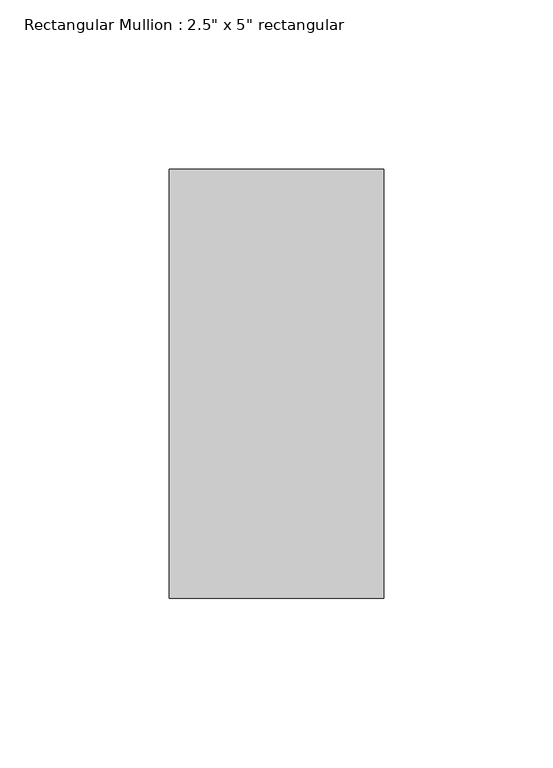
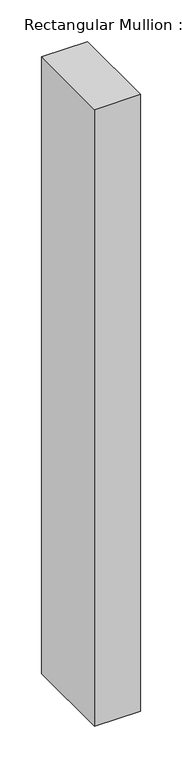
"""IFC4 building model written with IfcOpenShell, lengths in millimetres: member geometry."""

from ifc_helpers import new_model, si_unit, frame, origin, place, context, project, spatial, polyline, outline, extrude, source, transform, mapped, element, save


def member_b7368e82(model_context):
    return source(origin(), model_context, "Body", "SweptSolid", [
        extrude(outline(polyline([(0.0, 63.5), (0.0, -63.5), (-63.5, -63.5), (-63.5, 63.5), (0.0, 63.5)])), frame((0.0, 0.0, -901.7), z_axis=(0.0, 0.0, 1.0), x_axis=(1.0, 0.0, 0.0)), (0.0, 0.0, 1.0), 901.7),
    ])


if __name__ == "__main__":
    model = new_model("IFC4")
    model_context = context("Model", 3, world=origin())
    ifc_project = project(units=[si_unit("LENGTHUNIT", "METRE", prefix="MILLI")], contexts=[model_context])
    site = spatial("IfcSite", under=ifc_project)
    building = spatial("IfcBuilding", under=site)
    placement = place(None, origin())
    member_shape = member_b7368e82(model_context)
    element("IfcMember", 1, ObjectType="Rectangular Mullion : 2.5\" x 5\" rectangular", at=placement, inside=building, context=model_context, shape_type="MappedRepresentation", body=[
        mapped(member_shape, transform((0.0, 0.0, 0.0), x_axis=(1.0, 0.0, 0.0), y_axis=(0.0, 1.0, 0.0), z_axis=(0.0, 0.0, 1.0))),
    ])
    save(model, "model.ifc")

# Revit data of these elements
# Type "Rectangular Mullion : 2.5\" x 5\" rectangular"
#   built-in parameter 1007304 = 0.416667 (stored number, unit not read)
#   built-in parameter 1007301 = 0.104167 (stored number, unit not read)
#   built-in parameter 1007300 = 0.104167 (stored number, unit not read)
# Element 1 (IfcMember, "Rectangular Mullion : 2.5\" x 5\" rectangular")
#   Materials on its faces: "Aluminum"
# Materials
#   "Aluminum": class "Metal", colour RGB 247 247 247, transparency 0, Description = "Aluminum 6061", Cost = 0
